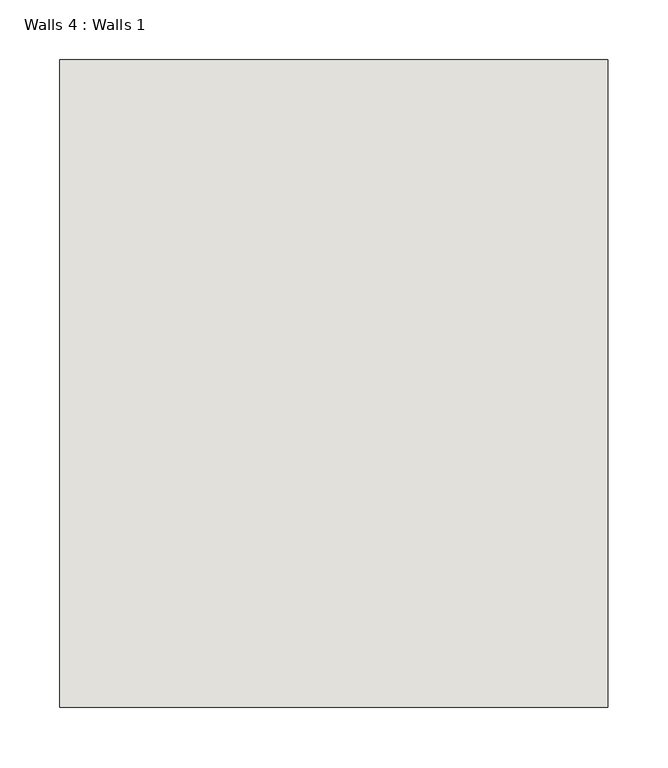
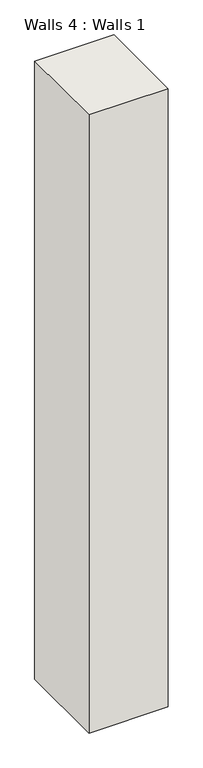
"""IFC4 building model written with IfcOpenShell, lengths in millimetres: wall geometry, Walls 4 : Walls 1."""

from ifc_helpers import new_model, si_unit, frame, origin, place, context, project, spatial, polyline, outline, extrude, source, transform, mapped, element, save


def walls_4_walls_1_0671908a(model_context):
    return source(origin(), model_context, "Body", "SweptSolid", [
        extrude(outline(polyline([(9864.6862424, -16395.9574082), (9407.4862424, -16395.9574082), (9407.4862424, -15855.5467593), (9864.6862424, -15855.5467593), (9864.6862424, -16395.9574082)])), frame((0.0, 0.0, 2895.6), z_axis=(0.0, 0.0, 1.0), x_axis=(1.0, 0.0, 0.0)), (0.0, 0.0, 1.0), 3769.177296),
    ])


if __name__ == "__main__":
    model = new_model("IFC4")
    model_context = context("Model", 3, world=origin())
    ifc_project = project(units=[si_unit("LENGTHUNIT", "METRE", prefix="MILLI")], contexts=[model_context])
    site = spatial("IfcSite", under=ifc_project)
    building = spatial("IfcBuilding", under=site)
    placement = place(None, origin())
    walls_4_walls_1_shape = walls_4_walls_1_0671908a(model_context)
    element("IfcWall", 1, ObjectType="Walls 4 : Walls 1", at=placement, inside=building, context=model_context, shape_type="MappedRepresentation", body=[
        mapped(walls_4_walls_1_shape, transform((0.0, 0.0, 0.0), x_axis=(1.0, 0.0, 0.0), y_axis=(0.0, 1.0, 0.0), z_axis=(0.0, 0.0, 1.0))),
    ])
    save(model, "model.ifc")

# Revit data of these elements
# Element 1 (IfcWall, "Walls 4 : Walls 1")
#   Materials on its faces: "WALL-2 GREY"
# Materials
#   "WALL-2 GREY": colour RGB 128 128 128, transparency 0, Cost = 0
